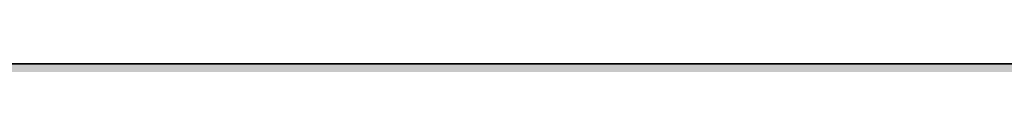
# Model space of a CAD drawing. Units: inches. Extents: x 2091 to 2899, y 967 to 2217.
# Tile 91 of 256: x 2251.31428 to 2251.38544, y 1099.91903 to 1099.91908. Entities that reach past the tile are written whole.
import ezdxf

# ---------------------------------------------------------------- set-up
doc = ezdxf.new("R2010")
doc.units = ezdxf.units.IN
doc.layers.add('A-WALL-PATT', color=141, linetype='Continuous', lineweight=13, true_color=0xadddf7)
doc.layers.add('L-SITE-WALL', color=7, linetype='Continuous', lineweight=35)

msp = doc.modelspace()

# ---------------------------------------------------------------- hatches: boundary and pattern name
at = {"layer": 'A-WALL-PATT'}
h = msp.add_hatch(color=256, dxfattribs=at)
h.dxf.hatch_style = 1
h.paths.add_polyline_path([(2212.143603, 1941.419059), (2387.643603, 1941.419059), (2387.643603, 1824.419059), (2392.143603, 1824.419059), (2392.143603, 1941.419059), (2609.643603, 1941.419059), (2609.643603, 1825.919059), (2614.143603, 1825.919059), (2614.143603, 1941.419059), (2794.143603, 1941.419059), (2794.143603, 1928.762166), (2803.143603, 1928.762166), (2803.143603, 2050.919059), (2203.143603, 2050.919059), (2203.143603, 1900.757859), (2212.143603, 1900.757859)])
h.paths.add_polyline_path([(2212.143603, 1945.919059), (2212.143603, 2041.919059), (2794.143603, 2041.919059), (2794.143603, 1945.919059), (2402.248245, 1945.919059), (2401.102434, 1945.775832), (2398.702434, 1945.775832)], flags=16)
h.paths.add_polyline_path([(2230.229861, 1948.062793), (2227.349861, 1949.502793), (2225.909861, 1951.902793), (2223.989861, 1952.862793), (2223.029861, 1955.262793), (2222.069861, 1959.582793), (2222.069861, 1963.422793), (2223.029861, 1965.662793), (2223.989861, 1965.342793), (2225.58591, 1963.860747), (2226.911533, 1964.957259), (2226.948861, 1965.938793), (2227.778319, 1966.952143), (2228.199916, 1968.878704), (2230.709861, 1964.862793), (2233.589861, 1966.302793), (2233.607309, 1966.331873), (2233.772659, 1964.938205), (2234.633802, 1963.676473), (2235.029861, 1963.902793), (2236.282035, 1965.572358), (2235.989861, 1962.942793), (2237.954512, 1957.540002), (2238.389861, 1957.902793), (2239.215861, 1960.305793), (2238.654565, 1966.38496), (2238.692792, 1966.438069), (2238.840578, 1967.499707), (2238.780291, 1967.687486), (2238.880538, 1967.786763), (2238.666861, 1966.251793), (2239.215861, 1960.305793), (2238.389861, 1957.902793), (2236.949861, 1956.702793), (2234.549861, 1949.982793)], flags=0)
h.paths.add_polyline_path([(2278.011974, 1948.062793), (2276.496427, 1947.873349), (2275.849833, 1947.688608), (2274.651974, 1947.102793)], flags=0)
h.paths.add_polyline_path([(2269.851974, 1955.742793), (2268.276176, 1956.629329), (2270.867302, 1956.348398), (2269.371974, 1958.142793), (2268.714964, 1959.192325), (2270.569833, 1958.728608), (2268.580725, 1961.906087), (2270.811974, 1960.891883), (2270.811974, 1963.422793), (2271.393315, 1964.779256), (2270.291762, 1966.156196), (2271.771974, 1965.662793), (2272.141387, 1966.524757), (2273.929833, 1965.928608), (2275.630385, 1968.054299), (2276.331938, 1966.72186), (2276.520431, 1966.952143), (2276.942029, 1968.878704), (2277.734293, 1967.611082), (2278.139888, 1969.46452), (2279.659124, 1967.033742), (2280.411974, 1966.782793), (2280.949302, 1967.588785), (2281.609833, 1967.368608), (2282.133266, 1968.153758), (2282.349235, 1966.333445), (2282.349849, 1966.332585), (2283.40755, 1968.09542), (2283.712631, 1965.52402), (2284.320221, 1964.633789), (2284.511809, 1964.889239), (2284.234974, 1965.704793), (2284.500472, 1967.318958), (2284.907944, 1965.41742), (2285.396313, 1966.068579), (2285.432833, 1966.290608), (2285.473338, 1966.171279), (2286.353919, 1967.345387), (2286.222007, 1966.158173), (2287.663492, 1968.080154), (2287.713974, 1968.442793), (2288.481599, 1969.016679), (2288.573993, 1968.728897), (2288.917461, 1969.06904), (2288.606833, 1966.837608), (2288.928726, 1963.35131), (2288.934974, 1963.356793), (2288.929731, 1963.340422), (2289.015281, 1962.413869), (2290.111223, 1963.875126), (2290.132833, 1963.942608), (2290.217672, 1964.017058), (2290.111223, 1963.875126), (2289.155833, 1960.891608), (2288.594036, 1959.257227), (2288.571974, 1959.102793), (2289.531974, 1960.542793), (2290.011974, 1962.462793), (2290.19184, 1962.642659), (2289.769833, 1959.688608), (2286.889833, 1957.288608), (2284.489833, 1950.568608), (2283.314658, 1950.046308), (2283.291974, 1949.982793), (2280.290059, 1948.648608), (2281.129833, 1948.648608), (2282.569833, 1948.168608), (2283.204726, 1948.062793), (2278.971974, 1948.062793), (2276.091974, 1949.502793), (2274.651974, 1951.902793), (2272.731974, 1952.862793)], flags=0)
h.paths.add_polyline_path([(2271.158868, 1958.021765), (2272.969833, 1955.848608), (2272.009833, 1960.168608), (2272.009833, 1964.008608), (2272.624426, 1965.442658), (2274.328023, 1963.860747), (2275.653646, 1964.957259), (2275.637743, 1964.53909), (2277.412231, 1966.006888), (2277.032974, 1965.156793), (2276.829924, 1964.975597), (2276.766012, 1963.295014), (2277.449635, 1962.66022), (2279.451974, 1964.862793), (2282.331974, 1966.302793), (2283.529833, 1966.888608), (2283.294512, 1966.770948), (2283.912993, 1963.8847), (2284.899249, 1964.448275), (2284.731974, 1962.942793), (2286.696625, 1957.540002), (2287.131974, 1957.902793), (2287.541913, 1959.095388), (2287.779395, 1958.442311), (2285.682738, 1956.695097), (2285.876503, 1959.795336), (2284.731974, 1962.942793), (2284.899249, 1964.448275), (2283.912993, 1963.8847), (2284.223833, 1962.434116), (2283.424365, 1963.605484), (2281.609833, 1962.568608), (2281.129833, 1960.168608), (2282.089833, 1956.328608), (2283.049833, 1952.968608), (2282.569833, 1950.568608), (2280.169833, 1948.648608), (2279.883316, 1948.791867), (2278.971974, 1948.062793), (2278.971974, 1949.022793), (2278.672313, 1949.397368), (2277.289833, 1950.088608), (2275.849833, 1952.488608), (2273.929833, 1953.448608), (2272.489833, 1954.888608), (2271.921647, 1954.888608), (2271.771974, 1955.262793)], flags=0)
h.paths.add_polyline_path([(2311.994146, 1955.742793), (2312.062717, 1955.674221), (2312.0551, 1955.7085)], flags=0)
h.paths.add_polyline_path([(2331.956146, 1963.951793), (2333.396146, 1965.391793), (2331.077146, 1963.356793), (2330.998603, 1963.111517)], flags=0)
h.paths.add_polyline_path([(2310.554146, 1954.302793), (2307.039807, 1956.279943), (2310.762903, 1955.876284), (2312.474146, 1953.822793), (2313.434146, 1951.422793), (2315.354146, 1950.462793), (2316.794146, 1948.062793), (2317.466146, 1947.726793), (2319.368691, 1947.964611), (2317.754146, 1949.982793), (2317.569531, 1950.610485), (2316.794146, 1951.902793), (2314.874146, 1952.862793), (2313.914146, 1955.262793), (2311.514146, 1958.142793), (2309.375489, 1961.559168), (2311.514146, 1960.337078), (2311.514146, 1961.982793), (2310.604672, 1963.119635), (2311.726605, 1962.47853), (2312.418332, 1964.09256), (2312.255964, 1964.29552), (2313.194146, 1963.982793), (2313.914146, 1965.662793), (2314.646778, 1965.418582), (2315.354146, 1966.302793), (2316.794146, 1967.742793), (2316.157435, 1966.946904), (2317.034111, 1965.28186), (2317.222604, 1965.512143), (2317.777048, 1968.045771), (2318.474111, 1966.72186), (2318.662604, 1966.952143), (2319.084201, 1968.878704), (2321.207049, 1965.482147), (2322.161419, 1966.913702), (2322.554146, 1966.782793), (2322.785988, 1967.130555), (2322.881646, 1966.324293), (2323.312041, 1965.72174), (2323.651289, 1965.891364), (2324.3965, 1967.133382), (2324.656945, 1964.938205), (2324.971986, 1964.476611), (2325.38728, 1967.001499), (2325.940813, 1964.418348), (2327.228929, 1966.135836), (2327.16632, 1965.572358), (2328.059139, 1966.762783), (2328.224576, 1966.247486), (2329.667971, 1967.67691), (2329.664576, 1967.687486), (2329.764823, 1967.786763), (2329.551146, 1966.251793), (2330.100146, 1960.305793), (2329.332814, 1958.07347), (2329.313065, 1957.935225), (2329.634146, 1958.202793), (2330.234146, 1959.102793), (2330.714146, 1961.022793), (2331.034146, 1961.342793), (2330.714146, 1959.102793), (2329.634146, 1958.202793), (2329.274146, 1957.662793), (2327.712112, 1956.361098), (2325.434146, 1949.982793), (2324.333769, 1949.493736), (2323.994146, 1948.542793), (2319.674146, 1946.622793), (2316.794146, 1948.062793), (2315.354146, 1950.462793), (2313.434146, 1951.422793)], flags=0)
h.paths.add_polyline_path([(2321.335684, 1947.952023), (2321.114146, 1948.062793), (2321.114146, 1949.022793), (2319.194146, 1951.422793), (2316.794146, 1959.582793), (2316.663237, 1959.582793), (2315.354146, 1958.142793), (2314.394146, 1958.142793), (2313.148303, 1958.709085), (2312.954146, 1959.582793), (2312.954146, 1960.891883), (2315.834146, 1959.582793), (2316.663237, 1959.582793), (2317.314709, 1960.299412), (2315.030195, 1962.420747), (2316.355818, 1963.517259), (2316.372337, 1963.951615), (2316.470195, 1963.860747), (2317.795818, 1964.957259), (2317.755219, 1963.889687), (2319.175146, 1965.156793), (2319.498407, 1965.881372), (2321.114146, 1965.342793), (2323.235885, 1962.372358), (2325.686349, 1963.772623), (2325.542789, 1962.480576), (2325.198783, 1963.494014), (2324.47851, 1963.082429), (2324.926005, 1960.994116), (2324.078087, 1962.236473), (2322.414791, 1961.286018), (2322.074146, 1959.582793), (2323.034146, 1955.742793), (2323.994146, 1952.382793), (2323.514146, 1949.982793), (2322.142717, 1948.88565), (2322.074146, 1948.542793)], flags=0)
h.paths.add_polyline_path([(2320.207479, 1963.337459), (2320.154146, 1963.422793), (2320.394146, 1963.542793)], flags=0)
h.paths.add_polyline_path([(2353.850527, 1965.8105), (2354.030527, 1965.7505), (2354.330527, 1966.4505), (2354.330527, 1966.9305)], flags=0)
h.paths.add_polyline_path([(2359.020582, 1969.026412), (2359.098382, 1968.901932), (2359.233527, 1969.5195), (2359.233527, 1969.9995)], flags=0)
h.paths.add_polyline_path([(2358.256694, 1966.681672), (2357.983601, 1966.348035), (2358.211267, 1966.146175), (2358.410492, 1966.389568)], flags=0)
h.paths.add_polyline_path([(2357.768473, 1966.058778), (2357.7322, 1965.104967), (2357.751047, 1965.120556), (2357.769527, 1965.6065), (2357.769527, 1966.057843)], flags=0)
h.paths.add_polyline_path([(2359.111527, 1965.3045), (2359.111527, 1964.8245), (2359.844527, 1966.4675), (2359.844527, 1966.9475)], flags=0)
h.paths.add_polyline_path([(2360.223684, 1966.621449), (2360.698527, 1969.3625), (2360.698527, 1969.8425), (2360.210527, 1967.0255), (2360.210527, 1966.6425)], flags=0)
h.paths.add_polyline_path([(2363.450527, 1967.8905), (2363.450527, 1968.3705), (2362.490527, 1966.9305), (2362.656045, 1966.698776)], flags=0)
h.paths.add_polyline_path([(2364.475523, 1966.078826), (2365.850527, 1968.3705), (2365.850527, 1968.8505), (2364.427975, 1966.479581)], flags=0)
h.paths.add_polyline_path([(2366.313527, 1965.8525), (2366.366709, 1965.695829), (2366.802527, 1968.3455), (2366.802527, 1968.8255)], flags=0)
h.paths.add_polyline_path([(2367.16531, 1965.803544), (2367.290527, 1966.9305), (2367.290527, 1967.4105), (2367.102701, 1965.720066)], flags=0)
h.paths.add_polyline_path([(2370.036527, 1959.9735), (2371.013527, 1963.0245), (2371.013527, 1963.5045), (2370.036527, 1960.4535)], flags=0)
h.paths.add_polyline_path([(2371.610527, 1960.2105), (2372.570527, 1961.6505), (2372.570527, 1962.1305), (2371.802527, 1960.9785)], flags=0)
h.paths.add_polyline_path([(2350.873666, 1956.005086), (2351.930527, 1955.8905), (2354.490527, 1953.3305), (2353.850527, 1954.9305), (2351.450527, 1957.8105), (2347.935527, 1963.4255), (2347.935527, 1963.9055), (2351.450527, 1958.2905), (2353.705073, 1955.585046), (2352.890527, 1959.2505), (2352.890527, 1959.7305), (2352.890527, 1961.924786), (2356.730527, 1959.7305), (2358.454471, 1961.626838), (2354.810527, 1965.0105), (2355.030855, 1965.28591), (2358.691091, 1961.88712), (2361.530527, 1965.0105), (2364.376495, 1966.433484), (2364.524394, 1965.186911), (2365.454468, 1963.824181), (2365.881073, 1964.067955), (2365.370527, 1966.4505), (2365.370527, 1966.9305), (2366.810527, 1960.2105), (2366.810527, 1959.7305), (2366.388709, 1952.981409), (2367.770527, 1956.8505), (2368.641225, 1957.576082), (2366.810527, 1962.6105), (2366.810527, 1963.0905), (2368.775179, 1957.68771), (2369.210527, 1958.0505), (2370.001592, 1960.351867), (2369.475232, 1966.052668), (2369.513458, 1966.105777), (2369.514173, 1966.110912), (2369.475232, 1966.532668), (2369.513458, 1966.585777), (2369.614635, 1967.312591), (2369.182527, 1968.6585), (2369.182527, 1969.1385), (2369.600957, 1967.835194), (2369.701204, 1967.934471), (2369.717947, 1968.054743), (2370.145176, 1968.374145), (2369.778707, 1968.011224), (2369.701204, 1967.454471), (2370.468161, 1968.214004), (2369.674936, 1967.265771), (2369.514173, 1966.110912), (2370.036527, 1960.4535), (2370.036527, 1959.9735), (2369.441756, 1958.243191), (2370.650527, 1959.2505), (2371.045821, 1962.017559), (2371.130527, 1962.1305), (2370.650527, 1958.7705), (2367.770527, 1956.3705), (2365.370527, 1949.6505), (2362.079099, 1948.187643), (2363.450527, 1947.7305), (2361.050527, 1947.7305), (2360.090527, 1947.7305), (2357.103861, 1947.357167), (2360.090527, 1948.2105), (2358.170527, 1949.1705), (2356.730527, 1951.5705), (2354.810527, 1952.5305), (2351.930527, 1955.4105)], flags=0)
h.paths.add_polyline_path([(2361.050527, 1948.6905), (2359.130527, 1951.0905), (2356.730527, 1959.2505), (2355.770527, 1959.2505), (2352.890527, 1960.559591), (2352.890527, 1961.444786), (2355.890527, 1959.7305), (2356.730527, 1959.7305), (2356.837194, 1959.367834), (2361.530527, 1964.5305), (2363.248422, 1965.389448), (2364.92531, 1963.041805), (2362.490527, 1961.6505), (2362.063861, 1959.517167), (2362.970527, 1955.8905), (2363.930527, 1952.5305), (2363.930527, 1952.0505), (2363.450527, 1949.6505), (2361.050527, 1947.7305)], flags=0)
h.paths.add_polyline_path([(2359.130527, 1951.5705), (2359.290527, 1951.3705), (2361.050527, 1954.4505), (2361.050527, 1954.9305)], flags=0)
h.paths.add_polyline_path([(2357.219527, 1966.5455), (2356.792527, 1968.8145), (2356.792527, 1969.2945), (2357.219527, 1967.0255)], flags=0)
h.paths.add_polyline_path([(2361.050527, 1954.4505), (2361.530527, 1958.7705), (2361.530527, 1959.2505), (2361.050527, 1954.9305)], flags=0)
h.paths.add_polyline_path([(2402.548287, 1948.486076), (2402.302434, 1948.415832), (2402.590434, 1948.415832)], flags=0)
h.paths.add_polyline_path([(2394.142434, 1956.095832), (2395.685052, 1954.553214), (2396.720495, 1953.970679), (2396.062434, 1955.615832), (2395.241381, 1956.601096), (2395.878904, 1956.441715), (2395.102434, 1959.935832), (2395.102434, 1963.775832), (2396.062434, 1966.015832), (2397.022434, 1965.695832), (2398.618483, 1964.213787), (2399.944106, 1965.310299), (2399.981434, 1966.291832), (2400.810891, 1967.305183), (2401.232489, 1969.231744), (2403.537949, 1965.543008), (2403.941984, 1967.389316), (2404.702434, 1967.135832), (2405.460328, 1966.07478), (2406.622434, 1966.655832), (2406.639882, 1966.684913), (2406.805232, 1965.291245), (2406.925694, 1965.114746), (2407.342434, 1964.975832), (2407.874326, 1965.77367), (2408.1691, 1964.398055), (2409.314608, 1965.925398), (2409.217458, 1965.051054), (2409.445232, 1963.131245), (2410.306374, 1961.869513), (2410.702434, 1962.095832), (2411.442269, 1963.082279), (2411.165434, 1963.897832), (2411.616426, 1966.639757), (2411.725365, 1966.791109), (2411.873151, 1967.852747), (2411.812864, 1968.040526), (2411.913111, 1968.139803), (2411.699434, 1966.604832), (2412.248434, 1960.658832), (2413.225434, 1963.709832), (2414.3779, 1964.72116), (2414.513151, 1965.692747), (2414.452864, 1965.880526), (2414.553111, 1965.979803), (2414.3779, 1964.72116), (2414.519817, 1964.845697), (2414.365365, 1964.631109), (2414.339434, 1964.444832), (2414.888434, 1958.498832), (2414.062434, 1956.095832), (2412.622434, 1954.895832), (2410.17137, 1948.032854), (2410.016719, 1948.084404), (2405.902434, 1946.255832), (2405.902434, 1947.215832), (2405.204252, 1948.08856), (2404.222434, 1948.415832), (2403.262434, 1948.415832), (2400.382434, 1949.855832), (2399.662434, 1951.055832), (2397.982434, 1952.735832), (2397.022434, 1953.215832), (2395.685052, 1954.553214), (2392.656776, 1956.256908)], flags=0)
h.paths.add_polyline_path([(2409.08565, 1964.407441), (2409.130363, 1964.275715), (2409.262434, 1964.495832)], flags=0)
h.paths.add_polyline_path([(2397.742434, 1961.615832), (2398.702434, 1963.855832), (2399.662434, 1963.535832), (2401.426563, 1965.740994), (2401.791415, 1966.5588), (2402.071434, 1965.070832), (2402.835507, 1964.393367), (2403.262398, 1964.9149), (2403.338119, 1964.771086), (2402.615516, 1963.976223), (2402.498612, 1960.902238), (2403.542997, 1959.932452), (2404.413203, 1960.889679), (2404.702434, 1962.335832), (2407.916347, 1964.172354), (2409.520211, 1961.926944), (2410.987085, 1957.893042), (2411.422434, 1958.255832), (2412.047964, 1960.075625), (2412.410341, 1959.079088), (2411.675621, 1958.466821), (2411.662434, 1958.255832), (2411.62607, 1958.425529), (2409.982434, 1957.055832), (2407.582434, 1950.335832), (2403.262434, 1948.415832), (2403.262434, 1949.375832), (2401.342434, 1951.775832), (2399.416508, 1958.323981), (2397.742434, 1959.084923), (2397.742434, 1959.970118), (2397.102434, 1960.335832), (2397.742434, 1960.044923)], flags=0)
h.paths.add_polyline_path([(2405.902434, 1952.975832), (2405.950434, 1953.407832), (2406.016719, 1953.175832)], flags=0)
h.paths.add_polyline_path([(2449.817778, 1967.114014), (2449.752323, 1967.135832), (2449.793703, 1967.077901)], flags=0)
h.paths.add_polyline_path([(2451.697696, 1966.61812), (2451.740895, 1966.690118), (2451.692051, 1966.665696)], flags=0)
h.paths.add_polyline_path([(2454.343628, 1965.737572), (2455.752323, 1967.615832), (2455.992323, 1968.095832), (2454.364497, 1965.925398)], flags=0)
h.paths.add_polyline_path([(2457.547323, 1968.863832), (2457.787323, 1969.343832), (2457.054323, 1968.795832), (2457.007622, 1968.460345)], flags=0)
h.paths.add_polyline_path([(2456.921784, 1967.856662), (2456.802238, 1968.229016), (2456.723, 1967.659803)], flags=0)
h.paths.add_polyline_path([(2457.302323, 1967.376832), (2457.542323, 1967.856832), (2456.810323, 1966.839832), (2456.740516, 1966.700218), (2456.749021, 1966.608105)], flags=0)
h.paths.add_polyline_path([(2458.275323, 1963.709832), (2458.155343, 1963.335153), (2460.354323, 1965.264832), (2460.594323, 1965.744832)], flags=0)
h.paths.add_polyline_path([(2458.392323, 1962.815832), (2458.364088, 1962.618185), (2459.592323, 1964.255832), (2459.832323, 1964.735832)], flags=0)
h.paths.add_polyline_path([(2459.352323, 1962.815832), (2459.272323, 1962.495832), (2460.072323, 1963.295832), (2460.312323, 1963.775832)], flags=0)
h.paths.add_polyline_path([(2458.680323, 1960.607832), (2458.632323, 1960.415832), (2459.592323, 1961.855832), (2459.832323, 1962.335832)], flags=0)
h.paths.add_polyline_path([(2437.83817, 1956.24265), (2439.192323, 1956.095832), (2441.352323, 1953.935832), (2440.872323, 1955.135832), (2438.472323, 1958.015832), (2438.071563, 1958.656023), (2438.712323, 1958.495832), (2440.639596, 1956.183105), (2439.912323, 1959.455832), (2439.912323, 1963.295832), (2441.352323, 1966.655832), (2441.592323, 1967.135832), (2441.112323, 1966.015832), (2442.072323, 1965.695832), (2443.988993, 1968.09167), (2444.241323, 1966.750832), (2444.916801, 1966.15192), (2445.676574, 1967.080136), (2446.255323, 1969.724832), (2446.495323, 1970.204832), (2446.282379, 1969.231744), (2447.362672, 1967.503275), (2447.720323, 1969.567832), (2447.960323, 1970.047832), (2447.48548, 1967.306781), (2448.792323, 1965.215832), (2448.472323, 1964.863832), (2448.552323, 1964.735832), (2451.452051, 1966.185696), (2451.615122, 1964.811245), (2452.307917, 1963.796172), (2453.234505, 1964.325651), (2454.072323, 1960.415832), (2453.628687, 1953.317651), (2454.792323, 1956.575832), (2455.032323, 1957.055832), (2455.718835, 1957.627926), (2453.832323, 1962.815832), (2453.940966, 1963.793615), (2453.335323, 1965.577832), (2453.824323, 1968.550832), (2454.064323, 1969.030832), (2453.575323, 1966.057832), (2454.040333, 1964.687919), (2453.832323, 1962.815832), (2455.718835, 1957.627926), (2456.367207, 1958.168235), (2457.058323, 1960.178832), (2457.298323, 1960.658832), (2456.472323, 1958.255832), (2457.717729, 1959.29367), (2457.672323, 1958.975832), (2454.889951, 1956.657188), (2453.614142, 1953.084923), (2453.592323, 1952.735832), (2453.352323, 1952.255832), (2453.359596, 1952.372196), (2452.632323, 1950.335832), (2452.392323, 1949.855832), (2449.203752, 1948.43869), (2450.712323, 1947.935832), (2448.072323, 1947.935832), (2447.112323, 1947.935832), (2444.552323, 1947.615832), (2447.199596, 1948.372196), (2445.192323, 1949.375832), (2443.752323, 1951.775832), (2441.832323, 1952.735832), (2438.952323, 1955.615832)], flags=0)
h.paths.add_polyline_path([(2443.992323, 1959.935832), (2444.040323, 1959.772632), (2444.121554, 1959.861986)], flags=0)
h.paths.add_polyline_path([(2442.912323, 1959.935832), (2443.032323, 1959.935832), (2442.445657, 1960.202499)], flags=0)
h.paths.add_polyline_path([(2444.982943, 1965.019677), (2445.279323, 1965.264832), (2445.519323, 1965.744832), (2444.993996, 1965.310299)], flags=0)
h.paths.add_polyline_path([(2446.133323, 1965.029832), (2446.330366, 1965.471499), (2444.970323, 1964.257832), (2444.730323, 1963.777832)], flags=0)
h.paths.add_polyline_path([(2442.792323, 1959.455832), (2443.752323, 1959.455832), (2446.152323, 1951.295832), (2446.412323, 1951.750832), (2446.392323, 1951.775832), (2448.080599, 1954.730315), (2448.552323, 1958.975832), (2441.832323, 1965.215832), (2442.154946, 1965.619111), (2448.792323, 1959.455832), (2448.312323, 1955.135832), (2448.072323, 1954.655832), (2446.412323, 1951.750832), (2448.312323, 1949.375832), (2448.312323, 1948.415832), (2450.540895, 1950.19869), (2450.952323, 1952.255832), (2449.992323, 1955.615832), (2449.032323, 1959.455832), (2449.512323, 1961.855832), (2449.752323, 1962.335832), (2449.674904, 1961.948736), (2452.994505, 1963.845651), (2453.064414, 1963.519409), (2452.884611, 1963.782854), (2449.674904, 1961.948736), (2449.272323, 1959.935832), (2450.232323, 1956.095832), (2451.192323, 1952.735832), (2450.712323, 1950.335832), (2450.472323, 1949.855832), (2448.072323, 1947.935832), (2448.072323, 1948.535832), (2445.432323, 1949.855832), (2443.992323, 1952.255832), (2442.072323, 1953.215832), (2441.112323, 1955.615832), (2440.152323, 1959.935832), (2440.152323, 1960.655832)], flags=0)
h.paths.add_polyline_path([(2456.692323, 1966.985832), (2457.608323, 1968.080832), (2457.848323, 1968.560832), (2456.932323, 1967.465832)], flags=0)
h.paths.add_polyline_path([(2489.89657, 1966.580241), (2489.942948, 1966.189347), (2490.747488, 1967.530248), (2491.319122, 1968.951161)], flags=0)
h.paths.add_polyline_path([(2473.562471, 1956.407131), (2477.139981, 1956.019257), (2476.955333, 1956.240834), (2475.108049, 1957.280108), (2476.347488, 1956.970248), (2475.186901, 1958.824216), (2476.919122, 1958.391161), (2475.411642, 1960.799269), (2477.787488, 1959.719339), (2477.787488, 1962.250248), (2477.637399, 1962.43786), (2477.82255, 1962.332059), (2478.359122, 1963.58406), (2478.359122, 1963.671161), (2477.324348, 1964.964628), (2478.714826, 1964.501135), (2479.319122, 1965.911161), (2480.279122, 1965.591161), (2481.783965, 1967.472214), (2482.116488, 1965.705248), (2482.880562, 1965.027782), (2483.209305, 1965.429408), (2483.220169, 1965.71509), (2483.07594, 1965.989022), (2483.711762, 1966.765808), (2484.130488, 1968.679248), (2484.702122, 1970.100161), (2484.489177, 1969.127072), (2486.502904, 1965.905109), (2487.387488, 1965.610248), (2488.153419, 1966.759144), (2488.717017, 1965.970108), (2489.200086, 1966.211642), (2489.330671, 1965.110992), (2490.393905, 1963.622465), (2490.660765, 1963.774956), (2490.493905, 1964.553636), (2490.923063, 1963.924841), (2491.319122, 1964.151161), (2491.333389, 1964.170183), (2491.210488, 1964.532248), (2491.281756, 1964.965537), (2491.425789, 1964.293383), (2494.076476, 1967.827632), (2494.497918, 1966.514942), (2494.598165, 1966.614218), (2494.689488, 1967.270248), (2495.106748, 1967.582196), (2495.129839, 1967.748075), (2495.069552, 1967.935854), (2495.169799, 1968.035131), (2495.031777, 1967.043632), (2495.753818, 1967.758684), (2494.982053, 1966.686437), (2494.956122, 1966.500161), (2495.479021, 1960.836851), (2495.910488, 1962.184248), (2496.482122, 1963.605161), (2496.072694, 1962.326589), (2496.768904, 1962.937536), (2496.599122, 1962.711161), (2496.119122, 1959.351161), (2496.732873, 1960.271787), (2496.987488, 1961.290248), (2497.559122, 1962.711161), (2497.079122, 1960.791161), (2496.507488, 1959.370248), (2495.547488, 1957.930248), (2492.758842, 1955.606376), (2490.839122, 1950.231161), (2490.267488, 1948.810248), (2485.947488, 1946.890248), (2483.067488, 1948.330248), (2481.627488, 1950.730248), (2479.707488, 1951.690248), (2476.827488, 1954.570248)], flags=0)
h.paths.add_polyline_path([(2485.576973, 1948.313392), (2485.559122, 1948.311161), (2485.578758, 1948.311161)], flags=0)
h.paths.add_polyline_path([(2478.645063, 1954.551161), (2478.109042, 1956.963257), (2479.319122, 1955.511161), (2480.279122, 1953.111161), (2482.199122, 1952.151161), (2483.639122, 1949.751161), (2486.519122, 1948.311161), (2486.519122, 1949.271161), (2484.739307, 1951.49593), (2484.027488, 1950.250248), (2481.627488, 1958.410248), (2482.375148, 1959.232673), (2482.199122, 1959.831161), (2483.197572, 1960.929456), (2479.707488, 1964.170248), (2480.603358, 1965.290085), (2481.875171, 1964.109115), (2482.666387, 1964.763582), (2482.615359, 1963.421798), (2482.989199, 1963.074661), (2484.008488, 1963.984248), (2484.683606, 1965.497507), (2484.580122, 1965.405161), (2485.357268, 1967.147113), (2485.120645, 1965.781197), (2486.427488, 1963.690248), (2488.145383, 1964.549195), (2489.822271, 1962.201552), (2490.747488, 1962.730248), (2491.999662, 1964.399813), (2492.076046, 1965.087265), (2492.212892, 1964.684119), (2492.485374, 1965.047429), (2492.279122, 1963.191161), (2494.243773, 1957.78837), (2494.562503, 1958.053978), (2494.933488, 1959.133248), (2495.505122, 1960.554161), (2494.679122, 1958.151161), (2494.107488, 1956.730248), (2494.562503, 1958.053978), (2493.408544, 1957.092345), (2491.707488, 1961.770248), (2491.999662, 1964.399813), (2490.747488, 1962.730248), (2487.71203, 1960.9957), (2487.479122, 1959.831161), (2488.439122, 1955.991161), (2489.399122, 1952.631161), (2488.919122, 1950.231161), (2488.576918, 1949.957397), (2488.347488, 1948.810248), (2487.651715, 1948.253629), (2487.479122, 1948.311161), (2486.519122, 1948.311161), (2483.639122, 1949.751161), (2482.199122, 1952.151161), (2480.279122, 1953.111161), (2478.839122, 1954.551161)], flags=0)
h.paths.add_polyline_path([(2526.648252, 1966.987524), (2526.517343, 1967.031161), (2526.600102, 1966.915298)], flags=0)
h.paths.add_polyline_path([(2528.47064, 1966.446656), (2528.574486, 1966.619732), (2528.457071, 1966.561025)], flags=0)
h.paths.add_polyline_path([(2534.133343, 1967.496161), (2534.156685, 1967.542845), (2534.059841, 1967.408296)], flags=0)
h.paths.add_polyline_path([(2536.161923, 1964.0506), (2535.157343, 1962.711161), (2535.100872, 1962.315866), (2536.117343, 1963.671161), (2536.420532, 1964.277539)], flags=0)
h.paths.add_polyline_path([(2535.157343, 1959.831161), (2536.117343, 1961.271161), (2536.597343, 1962.231161), (2535.253343, 1960.215161)], flags=0)
h.paths.add_polyline_path([(2513.249035, 1956.284796), (2516.221181, 1955.962555), (2514.997343, 1957.431161), (2514.195823, 1958.711541), (2515.477343, 1958.391161), (2516.931888, 1956.645706), (2516.437343, 1958.871161), (2516.437343, 1962.711161), (2516.872692, 1963.726974), (2515.346434, 1965.634797), (2517.397343, 1964.951161), (2517.877343, 1966.071161), (2518.357343, 1967.031161), (2517.877343, 1965.911161), (2518.837343, 1965.591161), (2520.48659, 1967.652719), (2520.766343, 1966.166161), (2521.530417, 1965.488695), (2521.781443, 1965.795375), (2521.800911, 1966.307268), (2521.477804, 1966.920936), (2521.246343, 1967.126161), (2521.177701, 1967.490913), (2521.477804, 1966.920936), (2522.010417, 1966.448695), (2522.257386, 1966.750417), (2522.780343, 1969.140161), (2523.260343, 1970.100161), (2523.047398, 1969.127072), (2524.673132, 1966.525897), (2526.037343, 1966.071161), (2526.795238, 1965.010108), (2527.977071, 1965.601025), (2528.140141, 1964.226573), (2528.66459, 1963.458159), (2529.388616, 1963.871888), (2529.329665, 1964.14699), (2529.481284, 1963.924841), (2529.877343, 1964.151161), (2529.98401, 1964.293383), (2529.789053, 1965.20318), (2530.0624, 1964.397903), (2532.802483, 1968.051347), (2533.147773, 1966.975854), (2533.24802, 1967.075131), (2533.339343, 1967.731161), (2533.672848, 1967.980493), (2533.72802, 1968.035131), (2533.514343, 1966.500161), (2534.024718, 1960.972496), (2534.560343, 1962.645161), (2535.040343, 1963.605161), (2534.063343, 1960.554161), (2533.237343, 1958.151161), (2534.288154, 1959.026836), (2534.197343, 1958.391161), (2531.512597, 1956.153872), (2529.397343, 1950.231161), (2528.917343, 1949.271161), (2526.448772, 1948.174018), (2527.477343, 1947.831161), (2530.357343, 1947.351161), (2524.597343, 1947.351161), (2521.717343, 1948.791161), (2520.277343, 1951.191161), (2518.357343, 1952.151161), (2515.477343, 1955.031161)], flags=0)
h.paths.add_polyline_path([(2523.93476, 1967.190308), (2523.619512, 1966.483689), (2523.7705, 1966.242109)], flags=0)
h.paths.add_polyline_path([(2518.837343, 1953.111161), (2517.877343, 1955.511161), (2516.884983, 1959.976779), (2516.917343, 1959.96207), (2516.917343, 1962.025446), (2520.757343, 1959.831161), (2522.024949, 1961.225527), (2518.357343, 1964.631161), (2519.002589, 1965.437718), (2520.433392, 1964.109115), (2521.30112, 1964.826871), (2521.245157, 1963.355333), (2525.638307, 1959.27598), (2526.037343, 1961.271161), (2529.397343, 1963.191161), (2530.649517, 1964.860726), (2530.66472, 1964.99755), (2530.691956, 1964.917311), (2531.087778, 1965.445074), (2530.945985, 1964.168944), (2530.691956, 1964.917311), (2529.397343, 1963.191161), (2526.362504, 1961.456967), (2526.037343, 1959.831161), (2526.997343, 1955.991161), (2527.957343, 1952.631161), (2527.477343, 1950.231161), (2527.134486, 1949.956875), (2526.973928, 1949.154087), (2526.697343, 1949.031161), (2524.597343, 1947.351161), (2524.597343, 1948.311161), (2524.277343, 1948.711161), (2522.197343, 1949.751161), (2520.757343, 1952.151161)], flags=0)
h.paths.add_polyline_path([(2520.277343, 1958.871161), (2520.853343, 1959.504761), (2523.157343, 1951.671161), (2524.613895, 1954.220126), (2524.597343, 1954.071161), (2522.677343, 1950.711161)], flags=0)
h.paths.add_polyline_path([(2559.37091, 1966.311161), (2559.398411, 1966.324911), (2559.401943, 1966.345296)], flags=0)
h.paths.add_polyline_path([(2549.77091, 1957.191161), (2552.65091, 1954.311161), (2552.133987, 1955.603468), (2550.61091, 1957.431161), (2547.09591, 1963.046161), (2545.77591, 1965.206161), (2549.29091, 1959.591161), (2551.69091, 1956.711161), (2550.792933, 1960.752059), (2550.73091, 1960.780251), (2550.73091, 1964.871161), (2551.69091, 1967.111161), (2552.65091, 1966.791161), (2554.246959, 1965.309115), (2555.034252, 1965.960337), (2555.581671, 1966.644612), (2555.60991, 1967.387161), (2556.439368, 1968.400511), (2556.860966, 1970.327072), (2559.37091, 1966.311161), (2560.69091, 1964.151161), (2562.408805, 1965.010108), (2561.65091, 1966.071161), (2560.33091, 1968.231161), (2561.758497, 1966.23254), (2562.347213, 1967.115614), (2562.433709, 1966.386573), (2563.127798, 1965.369604), (2563.57091, 1965.591161), (2563.588359, 1965.620241), (2563.362543, 1967.52354), (2563.722489, 1965.843792), (2565.060001, 1968.072979), (2564.732862, 1965.128722), (2565.117577, 1963.333383), (2567.444622, 1966.436109), (2567.315615, 1967.833328), (2567.353841, 1967.886437), (2567.501627, 1968.948075), (2567.44134, 1969.135854), (2567.541587, 1969.235131), (2567.32791, 1967.700161), (2567.87691, 1961.754161), (2568.746689, 1964.470327), (2568.635615, 1965.673328), (2568.673841, 1965.726437), (2568.821627, 1966.788075), (2568.76134, 1966.975854), (2568.861587, 1967.075131), (2568.64791, 1965.540161), (2568.726127, 1964.693026), (2568.85391, 1964.805161), (2568.746689, 1964.470327), (2568.817236, 1963.706261), (2568.97091, 1963.911161), (2568.866075, 1963.17731), (2569.19691, 1959.594161), (2568.37091, 1957.191161), (2566.93091, 1955.991161), (2564.620272, 1949.521373), (2564.65091, 1949.511161), (2564.616625, 1949.511161), (2564.53091, 1949.271161), (2560.21091, 1947.351161), (2557.33091, 1948.791161), (2556.045196, 1950.934018), (2556.01091, 1950.951161), (2555.856625, 1951.208303), (2553.97091, 1952.151161), (2551.09091, 1955.031161), (2546.650144, 1957.529515)], flags=0)
h.paths.add_polyline_path([(2567.025794, 1959.33023), (2567.035007, 1959.304895), (2567.05091, 1959.351161)], flags=0)
h.paths.add_polyline_path([(2551.968287, 1962.518374), (2553.01091, 1964.951161), (2553.97091, 1964.631161), (2555.566959, 1963.149115), (2556.892583, 1964.245627), (2556.92991, 1965.227161), (2557.143984, 1965.488695), (2556.420066, 1966.130557), (2556.391421, 1966.104995), (2556.37991, 1966.166161), (2556.420066, 1966.130557), (2556.95191, 1966.605161), (2557.092139, 1966.919478), (2557.570875, 1966.010228), (2557.759368, 1966.240511), (2557.41791, 1964.680161), (2556.892583, 1964.245627), (2556.807089, 1961.997566), (2560.69091, 1958.391161), (2560.635526, 1957.892699), (2560.81091, 1957.191161), (2561.77091, 1953.831161), (2561.29091, 1951.431161), (2559.110423, 1949.68677), (2559.156484, 1949.629193), (2563.02652, 1951.349209), (2562.61091, 1949.271161), (2560.21091, 1947.351161), (2560.21091, 1948.311161), (2559.25091, 1949.511161), (2558.89091, 1949.511161), (2558.89091, 1949.961161), (2558.29091, 1950.711161), (2558.053701, 1951.517672), (2556.97091, 1952.871161), (2555.06788, 1959.341464), (2552.05091, 1961.065446), (2552.05091, 1962.471161)], flags=0)
h.paths.add_polyline_path([(2588.330049, 1958.391161), (2588.610248, 1958.110962), (2588.553362, 1958.366949)], flags=0)
h.paths.add_polyline_path([(2594.745454, 1950.493086), (2593.957532, 1953.172022), (2593.130049, 1954.551161), (2591.210049, 1955.511161), (2590.250049, 1957.911161), (2588.309033, 1960.240379), (2586.177306, 1961.209346), (2587.850049, 1960.791161), (2587.253416, 1961.744246), (2588.441314, 1961.065446), (2588.441314, 1962.655528), (2588.421679, 1962.665345), (2588.441314, 1962.711161), (2586.914038, 1964.620256), (2588.877086, 1963.727962), (2589.290049, 1964.69154), (2589.290049, 1966.071161), (2590.250049, 1968.311161), (2591.210049, 1967.991161), (2592.806098, 1966.509115), (2594.131721, 1967.605627), (2594.169049, 1968.587161), (2594.998506, 1969.600511), (2595.420104, 1971.527072), (2597.930049, 1967.511161), (2600.810049, 1968.951161), (2600.827497, 1968.980241), (2600.992847, 1967.586573), (2601.853989, 1966.324841), (2602.107143, 1966.4695), (2602.236354, 1967.255069), (2602.356715, 1966.693383), (2603.502223, 1968.220726), (2603.210049, 1965.591161), (2605.1747, 1960.18837), (2605.506891, 1960.465196), (2605.026019, 1965.673328), (2605.064245, 1965.726437), (2605.212031, 1966.788075), (2605.151744, 1966.975854), (2605.251991, 1967.075131), (2605.343314, 1967.731161), (2605.952905, 1968.186898), (2605.874753, 1969.033328), (2605.912979, 1969.086437), (2606.060766, 1970.148075), (2606.000479, 1970.335854), (2606.100725, 1970.435131), (2605.887049, 1968.900161), (2606.436049, 1962.954161), (2605.610049, 1960.551161), (2605.997036, 1960.87365), (2606.564314, 1962.645161), (2608.241494, 1964.116941), (2608.010049, 1963.191161), (2607.050049, 1961.751161), (2606.631486, 1961.402358), (2606.201314, 1958.391161), (2603.321314, 1955.991161), (2600.921314, 1949.271161), (2596.601314, 1947.351161), (2593.721314, 1948.791161), (2592.857314, 1950.231161), (2592.650049, 1950.231161)], flags=0)
h.paths.add_polyline_path([(2596.601314, 1947.351161), (2596.601314, 1948.311161), (2594.681314, 1950.711161), (2596.154954, 1953.290029), (2595.530049, 1954.071161), (2593.199226, 1961.995957), (2592.65134, 1962.504708), (2591.780151, 1963.002531), (2593.282987, 1964.245627), (2593.320314, 1965.227161), (2594.149772, 1966.240511), (2594.57137, 1968.167072), (2596.182651, 1965.589023), (2596.951273, 1966.434508), (2598.041314, 1966.071161), (2598.799209, 1965.010108), (2599.961314, 1965.591161), (2599.978763, 1965.620241), (2600.144113, 1964.226573), (2601.005255, 1962.964841), (2601.401314, 1963.191161), (2602.653488, 1964.860726), (2602.361314, 1962.231161), (2603.792748, 1958.294719), (2601.977644, 1953.212427), (2601.946208, 1952.709453), (2599.468755, 1951.608363), (2599.001314, 1949.271161)], flags=0)
h.paths.add_polyline_path([(2597.561314, 1958.871161), (2597.670966, 1959.419419), (2597.595054, 1958.736204)], flags=0)
h.paths.add_polyline_path([(2623.666305, 1961.254375), (2625.519163, 1960.791161), (2624.965544, 1961.675533), (2627.199163, 1960.660251), (2627.199163, 1961.151161), (2626.959163, 1962.231161), (2626.959163, 1963.491161), (2625.582321, 1965.212213), (2626.959163, 1964.425446), (2626.959163, 1965.831161), (2626.869163, 1965.861161), (2627.919163, 1968.311161), (2628.879163, 1967.991161), (2630.475212, 1966.509115), (2631.800835, 1967.605627), (2631.838163, 1968.587161), (2632.667621, 1969.600511), (2633.089218, 1971.527072), (2635.599163, 1967.511161), (2638.479163, 1968.951161), (2638.496611, 1968.980241), (2638.661961, 1967.586573), (2639.176273, 1966.833011), (2639.780216, 1967.839582), (2640.02583, 1966.693383), (2641.171337, 1968.220726), (2640.879163, 1965.591161), (2641.114265, 1964.94463), (2641.411337, 1965.340726), (2641.308099, 1964.411586), (2642.843814, 1960.18837), (2643.279163, 1960.551161), (2644.084736, 1962.894736), (2643.783867, 1966.153328), (2643.806834, 1966.185237), (2643.600676, 1968.418053), (2643.522812, 1968.660581), (2643.72988, 1970.148075), (2643.669593, 1970.335854), (2643.76984, 1970.435131), (2643.556163, 1968.900161), (2643.600676, 1968.418053), (2643.909593, 1967.455854), (2644.00984, 1967.555131), (2643.811743, 1966.132079), (2644.105163, 1962.954161), (2644.238773, 1961.350836), (2644.719163, 1961.751161), (2645.032853, 1962.221695), (2645.322163, 1963.125161), (2646.07642, 1963.787047), (2645.032853, 1962.221695), (2644.345163, 1960.074161), (2643.519163, 1957.671161), (2642.079163, 1956.471161), (2639.719612, 1949.864419), (2639.875527, 1949.838433), (2635.359163, 1947.831161), (2632.479163, 1949.271161), (2631.039163, 1951.671161), (2629.119163, 1952.631161), (2628.159163, 1955.031161), (2625.759163, 1957.911161)], flags=0)
h.paths.add_polyline_path([(2627.816306, 1956.574018), (2627.373708, 1958.565706), (2626.376306, 1959.762589), (2627.199163, 1959.351161), (2627.373708, 1958.565706), (2627.919163, 1957.911161), (2628.879163, 1955.511161), (2630.799163, 1954.551161), (2632.239163, 1952.151161), (2633.315025, 1951.613229), (2631.039163, 1959.351161), (2631.49783, 1959.855694), (2630.799163, 1962.231161), (2631.449867, 1962.946935), (2630.715212, 1963.629115), (2632.040835, 1964.725627), (2632.078163, 1965.707161), (2632.292237, 1965.968695), (2631.705339, 1966.489067), (2633.136441, 1967.766144), (2633.329218, 1968.647072), (2634.674718, 1966.494272), (2635.208465, 1967.081393), (2636.799163, 1966.551161), (2637.676404, 1967.867023), (2638.993946, 1966.022465), (2639.705345, 1966.428979), (2641.119163, 1959.831161), (2640.930072, 1956.805706), (2639.439163, 1952.631161), (2638.227456, 1952.092624), (2637.759163, 1949.751161), (2635.359163, 1947.831161), (2635.359163, 1948.791161), (2633.439163, 1951.191161), (2633.315025, 1951.613229), (2632.239163, 1952.151161), (2630.799163, 1954.551161), (2628.879163, 1955.511161)], flags=0)
h.paths.add_polyline_path([(2637.759163, 1953.831161), (2637.279163, 1955.511161), (2636.319163, 1959.351161), (2636.799163, 1961.751161), (2639.233946, 1963.142465), (2637.557058, 1965.490108), (2638.738891, 1966.081025), (2638.901961, 1964.706573), (2639.763104, 1963.444841), (2636.799163, 1961.751161), (2636.532496, 1960.417827), (2637.039163, 1958.391161), (2637.999163, 1955.031161)], flags=0)
h.paths.add_polyline_path([(2668.567407, 1951.431161), (2667.607407, 1953.831161), (2665.207407, 1956.711161), (2662.293903, 1961.365307), (2665.447407, 1959.591161), (2666.647407, 1958.391161), (2666.647407, 1959.975161), (2666.058317, 1960.68207), (2666.647407, 1960.345446), (2666.647407, 1961.991161), (2666.70009, 1962.114087), (2666.407407, 1963.431161), (2666.407407, 1967.271161), (2667.367407, 1969.511161), (2668.327407, 1969.191161), (2669.923457, 1967.709115), (2671.24908, 1968.805627), (2671.286407, 1969.787161), (2672.115865, 1970.800511), (2672.537463, 1972.727072), (2675.047407, 1968.711161), (2677.927407, 1970.151161), (2677.944856, 1970.180241), (2678.110206, 1968.786573), (2678.971348, 1967.524841), (2679.367407, 1967.751161), (2680.619581, 1969.420726), (2680.327407, 1966.791161), (2682.292059, 1961.38837), (2682.727407, 1961.751161), (2683.358306, 1963.586571), (2683.232112, 1964.953328), (2683.270338, 1965.006437), (2683.393215, 1965.889138), (2683.359969, 1966.249215), (2683.357837, 1966.255854), (2683.359229, 1966.257232), (2682.992112, 1970.233328), (2683.030338, 1970.286437), (2683.178124, 1971.348075), (2683.117837, 1971.535854), (2683.218084, 1971.635131), (2683.004407, 1970.100161), (2683.359229, 1966.257232), (2683.458084, 1966.355131), (2683.393215, 1965.889138), (2683.413908, 1965.665023), (2684.42381, 1966.872275), (2683.553407, 1964.154161), (2683.358306, 1963.586571), (2683.793407, 1958.874161), (2682.967407, 1956.471161), (2681.527407, 1955.271161), (2680.109226, 1951.300251), (2680.084933, 1950.911573), (2679.976846, 1950.929587), (2679.127407, 1948.551161), (2674.807407, 1946.631161), (2671.927407, 1948.071161), (2670.487407, 1950.471161)], flags=0)
h.paths.add_polyline_path([(2671.935683, 1953.227023), (2671.687407, 1953.351161), (2670.247407, 1955.751161), (2668.327407, 1956.711161), (2667.356741, 1959.137827), (2669.527407, 1958.151161), (2670.487407, 1958.151161), (2671.479407, 1959.242361), (2670.684402, 1961.94538), (2668.889599, 1963.611982), (2667.307407, 1964.331161), (2668.567407, 1963.911161), (2668.830937, 1964.240572), (2670.247407, 1963.431161), (2672.42214, 1965.823367), (2672.777463, 1967.447072), (2673.234074, 1966.716494), (2674.411919, 1968.012124), (2673.980564, 1965.522109), (2675.287407, 1963.431161), (2675.554074, 1963.564494), (2675.932407, 1965.456161), (2676.247407, 1965.351161), (2677.005302, 1964.290108), (2678.167407, 1964.871161), (2679.607407, 1967.271161), (2680.327407, 1963.911161), (2680.306552, 1963.57748), (2680.347242, 1963.457607), (2680.859581, 1964.140726), (2680.567407, 1961.511161), (2681.103624, 1960.036566), (2678.887407, 1953.831161), (2677.092478, 1953.033414), (2677.687407, 1950.951161), (2677.207407, 1948.551161), (2674.807407, 1946.631161), (2674.807407, 1947.591161), (2672.887407, 1949.991161)], flags=0)
h.paths.add_polyline_path([(2673.98455, 1951.911161), (2674.567407, 1952.931161), (2674.567407, 1951.911161), (2676.967407, 1953.831161), (2677.447407, 1956.231161), (2676.487407, 1959.591161), (2676.247407, 1960.551161), (2679.729589, 1962.540979), (2680.059267, 1961.002484), (2679.211348, 1962.244841), (2676.247407, 1960.551161), (2676.487407, 1959.591161), (2677.447407, 1956.231161), (2676.967407, 1953.831161), (2674.567407, 1951.911161)], flags=0)
h.paths.add_polyline_path([(2707.479283, 1952.814651), (2706.519283, 1955.214651), (2705.559283, 1959.534651), (2705.559283, 1963.374651), (2706.519283, 1965.614651), (2707.479283, 1965.294651), (2709.075332, 1963.812605), (2710.400956, 1964.909117), (2710.438283, 1965.890651), (2711.267741, 1966.904001), (2711.689338, 1968.830563), (2714.199283, 1964.814651), (2717.079283, 1966.254651), (2717.096731, 1966.283731), (2717.262082, 1964.890063), (2718.123224, 1963.628331), (2718.519283, 1963.854651), (2719.771457, 1965.524216), (2719.479283, 1962.894651), (2721.443934, 1957.49186), (2721.879283, 1957.854651), (2722.705283, 1960.257651), (2722.143988, 1966.336818), (2722.182214, 1966.389928), (2722.33, 1967.451565), (2722.269713, 1967.639345), (2722.36996, 1967.738621), (2722.156283, 1966.203651), (2722.705283, 1960.257651), (2721.879283, 1957.854651), (2720.439283, 1956.654651), (2718.039283, 1949.934651), (2713.719283, 1948.014651), (2710.839283, 1949.454651), (2709.399283, 1951.854651)], flags=0)
h.paths.add_polyline_path([(2749.301231, 1952.814651), (2748.341231, 1955.214651), (2747.381231, 1959.534651), (2747.381231, 1963.374651), (2748.341231, 1965.614651), (2749.301231, 1965.294651), (2750.89728, 1963.812605), (2752.222903, 1964.909117), (2752.260231, 1965.890651), (2753.089688, 1966.904001), (2753.511286, 1968.830563), (2756.021231, 1964.814651), (2758.901231, 1966.254651), (2758.918679, 1966.283731), (2759.084029, 1964.890063), (2759.945171, 1963.628331), (2760.341231, 1963.854651), (2761.593405, 1965.524216), (2761.301231, 1962.894651), (2763.265882, 1957.49186), (2763.701231, 1957.854651), (2764.527231, 1960.257651), (2763.965935, 1966.336818), (2764.004161, 1966.389928), (2764.151948, 1967.451565), (2764.091661, 1967.639345), (2764.191907, 1967.738621), (2763.978231, 1966.203651), (2764.527231, 1960.257651), (2763.701231, 1957.854651), (2762.261231, 1956.654651), (2759.861231, 1949.934651), (2755.541231, 1948.014651), (2752.661231, 1949.454651), (2751.221231, 1951.854651)], flags=0)
h.paths.add_polyline_path([(2212.143603, 1819.934514), (2203.143603, 1819.934514), (2203.143603, 1739.979546), (2212.143603, 1739.979546), (2212.143603, 1780.919059), (2392.143603, 1780.919059), (2392.143603, 1783.919059), (2212.143603, 1783.919059)])
h.paths.add_polyline_path([(2803.143603, 1847.938821), (2794.143603, 1847.938821), (2794.143603, 1785.419059), (2609.643603, 1785.419059), (2493.875609, 1785.419059), (2493.875609, 1780.919059), (2609.643603, 1780.919059), (2794.143603, 1780.919059), (2794.143603, 1696.919059), (2609.375609, 1696.919059), (2609.375609, 1742.919059), (2604.875609, 1742.919059), (2604.875609, 1644.419059), (2609.375609, 1644.419059), (2609.375609, 1692.419059), (2794.143603, 1692.419059), (2794.143603, 1668.164737), (2803.143603, 1668.164737)])
h.paths.add_polyline_path([(2392.143603, 1740.419059), (2387.643603, 1740.419059), (2387.643603, 1629.419059), (2212.143603, 1629.419059), (2212.143603, 1659.156202), (2203.143603, 1659.156202), (2203.143603, 1494.089439), (2212.143603, 1494.089439), (2212.143603, 1627.919059), (2392.143603, 1627.919059)])
h.paths.add_polyline_path([(2457.875609, 1780.919059), (2453.375609, 1780.919059), (2453.375609, 1644.419059), (2568.875609, 1644.419059), (2568.875609, 1648.919059), (2457.875609, 1648.919059)])
h.paths.add_polyline_path([(2545.143603, 1591.919059), (2540.643603, 1591.919059), (2540.643603, 1567.919059), (2468.643603, 1567.919059), (2468.643603, 1627.919059), (2509.143603, 1627.919059), (2509.143603, 1632.419059), (2464.143603, 1632.419059), (2464.143603, 1563.419059), (2545.143603, 1563.419059)])
h.paths.add_polyline_path([(2268.643603, 1555.919059), (2212.143603, 1555.919059), (2212.143603, 1551.419059), (2268.643603, 1551.419059)], flags=17)
h.paths.add_polyline_path([(2212.143603, 1413.266094), (2203.143603, 1413.266094), (2203.143603, 1233.070405), (2212.143603, 1233.070405)])
h.paths.add_polyline_path([(2267.643603, 1351.919059), (2212.143603, 1351.919059), (2212.143603, 1347.419059), (2267.643603, 1347.419059)], flags=17)
h.paths.add_polyline_path([(2456.643603, 1489.419059), (2452.143603, 1489.419059), (2452.143603, 1351.919059), (2312.643603, 1351.919059), (2312.643603, 1347.419059), (2456.643603, 1347.419059)])
h.paths.add_polyline_path([(2472.370171, 1455.419059), (2467.870171, 1455.419059), (2467.870171, 1347.419059), (2472.370171, 1347.419059)])
h.paths.add_polyline_path([(2794.143603, 1351.919059), (2543.370171, 1351.919059), (2543.370171, 1347.419059), (2794.143603, 1347.419059)], flags=17)
h.paths.add_polyline_path([(2312.643603, 1347.419059), (2308.143603, 1347.419059), (2308.143603, 1302.161787), (2308.341966, 1302.164327), (2308.143603, 1298.169249), (2308.143603, 1275.419059), (2212.143603, 1275.419059), (2212.143603, 1270.919059), (2312.643603, 1270.919059)], flags=17)
h.paths.add_polyline_path([(2212.143603, 1152.24706), (2203.143603, 1152.24706), (2203.143603, 1090.919059), (2803.143603, 1090.919059), (2803.143603, 1392.713555), (2794.143603, 1392.713555), (2794.143603, 1143.419059), (2548.032447, 1143.419059), (2548.032447, 1138.919059), (2794.143603, 1138.919059), (2794.143603, 1099.919059), (2212.143603, 1099.919059)])
h.paths.add_polyline_path([(2471.532447, 1266.328529, 0.031658), (2467.032447, 1269.945786), (2467.032447, 1143.419059), (2471.532447, 1143.419059), (2471.532447, 1148.819059)], flags=17)
h.paths.add_polyline_path([(2803.143603, 1587.341392), (2794.143603, 1587.341392), (2794.143603, 1473.5369), (2803.143603, 1473.5369)])
h.paths.add_polyline_path([(2794.143603, 1536.419059), (2651.143603, 1536.419059), (2651.143603, 1531.919059), (2794.143603, 1531.919059)])
h.paths.add_polyline_path([(2614.143603, 1620.419059), (2609.643603, 1620.419059), (2609.643603, 1536.419059), (2614.143603, 1536.419059)])
h.paths.add_polyline_path([(2271.082728, 1964.317238), (2776.852968, 1964.317238), (2776.852968, 2037.169623), (2271.082728, 2037.169623)], flags=8)
h.paths.add_polyline_path([(2380.649285, 1536.824144), (2461.040809, 1536.824144), (2461.040809, 1554.652587), (2380.649285, 1554.652587)], flags=9)
h.paths.add_polyline_path([(2203.655038, 1608.815312), (2316.118439, 1608.815312), (2316.118439, 1621.918356), (2203.655038, 1621.918356)], flags=24)
h.paths.add_polyline_path([(2212.677255, 1313.504102), (2282.59152, 1313.504102), (2282.59152, 1322.745239), (2212.677255, 1322.745239)], flags=24)
h.paths.add_polyline_path([(2457.111976, 1114.778574), (2558.481581, 1114.778574), (2558.481581, 1142.219682), (2457.111976, 1142.219682)], flags=25)
h.paths.add_polyline_path([(2473.442337, 1273.010067), (2604.641226, 1273.010067), (2604.641226, 1318.346935), (2473.442337, 1318.346935)], flags=25)
h.paths.add_polyline_path([(2638.876302, 1626.977432), (2684.250367, 1627.976738), (2684.038483, 1637.597494), (2638.664417, 1636.598188)], flags=9)
h.paths.add_polyline_path([(2537.590554, 1453.793447), (2628.389547, 1453.793447), (2628.389547, 1475.344811), (2537.590554, 1475.344811)], flags=9)
h.paths.add_polyline_path([(2504.137638, 1714.632397), (2554.647187, 1714.632397), (2554.647187, 1730.237712), (2504.137638, 1730.237712)], flags=25)
h.paths.add_polyline_path([(2487.501181, 1575.651872), (2535.097121, 1575.651872), (2535.097121, 1598.377646), (2487.501181, 1598.377646)], flags=25)
h.paths.add_polyline_path([(2709.0994, 1735.710278), (2740.016601, 1735.710278), (2740.016601, 1749.937641), (2709.0994, 1749.937641)], flags=25)
h.paths.add_polyline_path([(2442.438424, 1792.171657), (2564.728835, 1792.171657), (2564.728835, 1842.000163), (2442.438424, 1842.000163)], flags=9)
h.paths.add_polyline_path([(2655.815801, 1809.644076), (2789.520142, 1806.693796), (2790.084977, 1832.291638), (2656.380635, 1835.241918)], flags=25)
h.paths.add_polyline_path([(2234.842697, 1797.720143), (2368.592851, 1794.768852), (2369.160718, 1820.504132), (2235.410564, 1823.455423)], flags=9)
h.paths.add_polyline_path([(2245.138466, 1644.006335), (2398.427733, 1640.6239), (2398.994842, 1666.32482), (2245.705575, 1669.707255)], flags=9)
h.paths.add_polyline_path([(2306.142847, 1431.168519), (2413.768314, 1428.793687), (2414.333148, 1454.391529), (2306.707682, 1456.76636)], flags=9)
h.paths.add_polyline_path([(2306.834582, 1458.233145), (2393.380484, 1456.323449), (2393.932808, 1481.354358), (2307.386907, 1483.264054)], flags=9)

# ---------------------------------------------------------------- linework, layer by layer
at = {"layer": 'L-SITE-WALL'}
msp.add_line((2794.143603, 1099.919059), (2212.143603, 1099.919059), dxfattribs=at)

doc.saveas('drawing.dxf')
